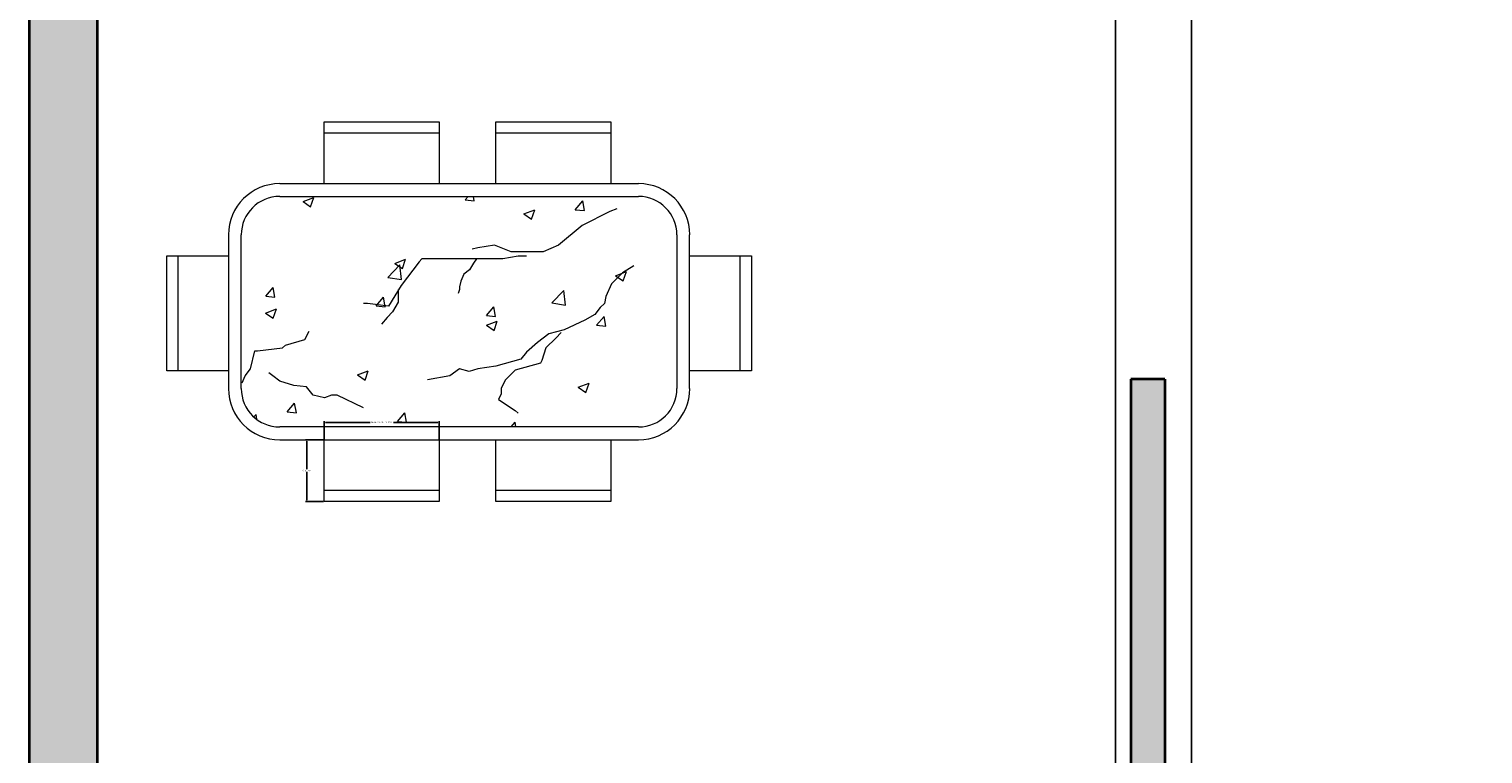
# Model space of a CAD drawing. Units: inches. Extents: x -5 to 366, y -496 to 54.
# Tile 8 of 10: x 22 to 214, y -205 to -110. Entities that reach past the tile are written whole.
import ezdxf

# ---------------------------------------------------------------- set-up
doc = ezdxf.new("R2010")
doc.units = ezdxf.units.IN
doc.header["$MEASUREMENT"] = 0
for name, color, linetype, lineweight in [('A-ANNO-DIMS', 2, 'Continuous', 18), ('A-FURN', 8, 'Continuous', 18), ('A-WALL', 7, 'Continuous', 35), ('A-WALL-PATT', 252, 'Continuous', 13)]:
    doc.layers.add(name, color=color, linetype=linetype, lineweight=lineweight)
doc.styles.get("Standard").update_dxf_attribs({"font": 'arial.ttf'})
doc.dimstyles.get("Standard").update_dxf_attribs({"dimtxt": 0.18, "dimasz": 0.18, "dimexe": 0.18, "dimexo": 0.0625, "dimgap": 0.09, "dimtad": 0, "dimtih": 1, "dimtoh": 1, "dimdec": 0, "dimzin": 0, "dimdsep": 46, "dimlunit": 3, "dimtxsty": 'Standard', "dimcen": 0.09, "dimadec": 0, "dimazin": 0, "dimtfac": 1, "dimtdec": 0, "dimtofl": 0, "dimtmove": 0, "dimatfit": 3, "dimfxl": 1, "dimtolj": 1, "dimtzin": 0, "dimarcsym": 0})

# ---------------------------------------------------------------- blocks, each defined once
blk = doc.blocks.new('CHAIR-DINING')
for p, q in [((0, 0), (0, 8.16)), ((0, 8.16), (15.22, 8.16)), ((15.22, 8.16), (15.22, 0)), ((15.22, 6.67), (0, 6.67))]:
    blk.add_line(p, q)
blk = doc.blocks.new('*D13')
at = {"layer": 'A-ANNO-DIMS', "color": 0, "lineweight": -2, "transparency": 16777216}
for p, q in [((60.89, -163.78), (60.89, -161.38)), ((61.07, -161.56), (66.97, -161.56)), ((75.93, -161.56), (70.04, -161.56)), ((76.11, -163.78), (76.11, -161.38))]:
    blk.add_line(p, q, dxfattribs=at)
at = {"layer": 'A-ANNO-DIMS', "color": 0, "transparency": 16777216}
for points in [[(61.07, -161.53), (61.07, -161.59), (60.89, -161.56)], [(75.93, -161.53), (75.93, -161.59), (76.11, -161.56)]]:
    blk.add_solid(points, dxfattribs=at)
at = {"layer": 'Defpoints', "color": 0, "transparency": 16777216}
for p in [(60.89, -161.56), (60.89, -163.84), (76.11, -163.84)]:
    blk.add_point(p, dxfattribs=at)
at = {"layer": 'A-ANNO-DIMS', "color": 0, "transparency": 16777216, "insert": (68.5, -161.56), "char_height": 0.18, "attachment_point": 5}
blk.add_mtext('\\A1;DINING CHAIR 1\'-3" TYP.', dxfattribs=at)
blk = doc.blocks.new('*D14')
at = {"layer": 'A-ANNO-DIMS', "color": 0, "lineweight": -2, "transparency": 16777216}
for p, q in [((60.83, -163.84), (58.42, -163.84)), ((58.6, -164.02), (58.6, -167.74)), ((58.6, -171.82), (58.6, -168.1)), ((60.83, -172), (58.42, -172))]:
    blk.add_line(p, q, dxfattribs=at)
at = {"layer": 'A-ANNO-DIMS', "color": 0, "transparency": 16777216}
for points in [[(58.57, -164.02), (58.63, -164.02), (58.6, -163.84)], [(58.57, -171.82), (58.63, -171.82), (58.6, -172)]]:
    blk.add_solid(points, dxfattribs=at)
at = {"layer": 'Defpoints', "color": 0, "transparency": 16777216}
for p in [(60.89, -163.84), (58.6, -172), (60.89, -172)]:
    blk.add_point(p, dxfattribs=at)
at = {"layer": 'A-ANNO-DIMS', "color": 0, "transparency": 16777216, "insert": (58.6, -167.92), "char_height": 0.18, "attachment_point": 5}
blk.add_mtext('\\A1;0\'-8" TYP.', dxfattribs=at)
blk = doc.blocks.new('*D29')
at = {"layer": 'A-ANNO-DIMS', "color": 0, "lineweight": -2, "transparency": 16777216}
for p, q in [((165.43, -380.42), (165.43, 53.15)), ((165.61, 52.97), (170.03, 52.97)), ((175.25, 52.97), (170.83, 52.97)), ((175.43, -380.42), (175.43, 53.15))]:
    blk.add_line(p, q, dxfattribs=at)
at = {"layer": 'A-ANNO-DIMS', "color": 0, "transparency": 16777216}
for points in [[(165.61, 53), (165.61, 52.94), (165.43, 52.97)], [(175.25, 53), (175.25, 52.94), (175.43, 52.97)]]:
    blk.add_solid(points, dxfattribs=at)
at = {"layer": 'Defpoints', "color": 0, "transparency": 16777216}
for p in [(175.43, 52.97), (165.43, -380.48), (175.43, -380.48)]:
    blk.add_point(p, dxfattribs=at)
at = {"layer": 'A-ANNO-DIMS', "color": 0, "transparency": 16777216, "insert": (170.43, 52.97), "char_height": 0.18, "attachment_point": 5}
blk.add_mtext('\\A1;0\'-10"', dxfattribs=at)

msp = doc.modelspace()

# ---------------------------------------------------------------- hatches: boundary and pattern name
at = {"layer": 'A-WALL-PATT'}
h = msp.add_hatch(color=256, dxfattribs=at)
h.dxf.hatch_style = 1
h.paths.add_polyline_path([(324.93, 26.52), (21.93, 26.52), (21.93, -456.98), (26.43, -456.98), (26.43, -331.98), (30.93, -331.98), (30.93, -322.98), (30.93, -106.98), (110.93, -106.98), (110.93, -104.73), (110.93, -102.48), (30.93, -102.48), (30.93, 17.52), (138.93, 17.52), (141.18, 17.52), (143.43, 17.52), (183.43, 17.52), (187.93, 17.52), (315.93, 17.52), (315.93, -102.48), (315.93, -106.98), (315.93, -255.48), (171.93, -255.48), (171.93, -155.84), (167.43, -155.84), (167.43, -291.98), (171.93, -291.98), (171.93, -259.98), (315.93, -259.98), (315.93, -375.98), (297.93, -375.98), (297.93, -380.48), (315.93, -380.48), (315.93, -452.48), (315.93, -456.98), (324.93, -456.98)])
h.paths.add_polyline_path([(143.43, -18.48), (143.43, -13.98), (138.93, -13.98), (138.93, -106.98), (187.93, -106.98), (187.93, -102.48), (143.43, -102.48)], flags=17)

# ---------------------------------------------------------------- linework, layer by layer
at = {"layer": 'A-FURN'}
for p, q in [((102.41, -130.01), (55.03, -130.01)), ((55.03, -131.7), (102.41, -131.7)), ((58.11, -132.38), (59.53, -131.83)), ((58.11, -132.38), (59.12, -133.06)), ((59.12, -133.06), (59.53, -131.83)), ((79.51, -132.16), (79.9, -131.7)), ((79.51, -132.16), (80.72, -132.27)), ((80.72, -132.27), (80.62, -131.7)), ((94.07, -133.44), (95.05, -132.27)), ((95.28, -133.55), (95.05, -132.27)), ((87.28, -134), (88.71, -133.46)), ((87.28, -134), (88.29, -134.68)), ((88.29, -134.68), (88.71, -133.46)), ((94.07, -133.44), (95.28, -133.54)), ((98.65, -133.7), (94.97, -135.54)), ((99.57, -133.34), (98.65, -133.7)), ((94.97, -135.54), (91.85, -138.11)), ((48.27, -136.77), (48.27, -157.08)), ((49.96, -157.08), (49.96, -136.77)), ((83.38, -138.11), (81.18, -138.48)), ((85.59, -139.03), (83.38, -138.11)), ((91.85, -138.11), (89.82, -139.03)), ((107.48, -136.77), (107.48, -157.08)), ((109.17, -157.08), (109.17, -136.77)), ((70.23, -140.55), (71.65, -140)), ((71.24, -141.23), (71.65, -140)), ((73.82, -139.95), (73.45, -140.32)), ((84.49, -139.95), (73.82, -139.95)), ((81.18, -138.48), (80.44, -138.67)), ((81, -139.94), (80.63, -140.5)), ((86.51, -139.58), (84.49, -139.95)), ((89.82, -139.03), (85.59, -139.03)), ((87.62, -139.58), (86.51, -139.58)), ((69.31, -142.39), (70.9, -140.75)), ((70.23, -140.55), (71.24, -141.23)), ((71.12, -142.68), (70.9, -140.75)), ((73.45, -140.32), (71.06, -143.44)), ((79.34, -141.97), (78.97, -142.88)), ((80.08, -141.41), (79.34, -141.97)), ((80.63, -140.5), (80.08, -141.41)), ((100.31, -141.79), (98.84, -143.26)), ((99.4, -142.18), (100.83, -141.63)), ((101.78, -140.87), (100.31, -141.79)), ((100.41, -142.86), (100.83, -141.63)), ((53.2, -144.89), (54.18, -143.72)), ((54.41, -145), (54.18, -143.72)), ((69.31, -142.39), (71.12, -142.67)), ((71.06, -143.44), (69.4, -146.2)), ((70.69, -143.99), (70.69, -145.65)), ((78.79, -143.99), (78.6, -144.54)), ((78.97, -142.88), (78.79, -143.62)), ((78.79, -143.62), (78.79, -143.99)), ((98.84, -143.26), (98.1, -144.91)), ((99.4, -142.18), (100.41, -142.86)), ((53.2, -144.89), (54.41, -144.99)), ((66.64, -145.83), (66.09, -145.83)), ((69.4, -146.2), (66.64, -145.83)), ((67.76, -146.16), (68.74, -145)), ((68.98, -146.27), (68.74, -145)), ((70.69, -145.65), (69.95, -146.93)), ((90.98, -145.76), (92.56, -144.11)), ((90.98, -145.76), (92.79, -146.04)), ((92.79, -146.04), (92.56, -144.11)), ((97.92, -145.83), (97.37, -146.38)), ((98.1, -144.91), (97.92, -145.83)), ((53.17, -147.1), (54.59, -146.55)), ((53.17, -147.1), (54.18, -147.78)), ((54.18, -147.78), (54.59, -146.55)), ((67.76, -146.16), (68.98, -146.27)), ((69.22, -147.67), (68.48, -148.59)), ((69.95, -146.93), (69.22, -147.67)), ((82.33, -147.44), (83.3, -146.27)), ((82.33, -147.44), (83.54, -147.54)), ((83.54, -147.54), (83.3, -146.27)), ((96.63, -147.3), (95.34, -148.04)), ((97.37, -146.38), (96.63, -147.3)), ((96.89, -148.71), (97.87, -147.54)), ((98.1, -148.82), (97.87, -147.54)), ((58.36, -150.61), (58.92, -149.51)), ((82.35, -148.72), (83.77, -148.18)), ((82.35, -148.72), (83.35, -149.4)), ((83.36, -149.41), (83.77, -148.18)), ((92.58, -149.32), (90.56, -149.87)), ((92.21, -149.69), (91.48, -150.43)), ((95.34, -148.04), (92.58, -149.32)), ((96.89, -148.71), (98.1, -148.82)), ((55.42, -151.71), (55.79, -151.34)), ((55.79, -151.34), (58.36, -150.61)), ((89.09, -150.98), (87.62, -152.26)), ((90.56, -149.87), (89.09, -150.98)), ((91.48, -150.43), (90.19, -151.71)), ((51.19, -154.47), (51.74, -152.08)), ((51.74, -152.08), (52.11, -152.08)), ((52.11, -152.08), (55.42, -151.71)), ((86.88, -153.18), (83.57, -154.1)), ((87.62, -152.26), (86.88, -153.18)), ((89.64, -153.37), (89.46, -153.73)), ((90.19, -151.71), (89.64, -153.37)), ((50.09, -156.31), (50.45, -155.39)), ((50.45, -155.39), (51.19, -154.47)), ((54.14, -155.38), (53.58, -155.01)), ((55.06, -156.12), (54.14, -155.38)), ((65.29, -155.27), (66.71, -154.73)), ((65.29, -155.27), (66.3, -155.95)), ((66.3, -155.95), (66.71, -154.73)), ((77.5, -155.39), (74.55, -155.94)), ((78.79, -154.47), (77.5, -155.39)), ((80.07, -154.84), (78.79, -154.47)), ((81.18, -154.47), (80.07, -154.84)), ((83.57, -154.1), (81.18, -154.47)), ((86.14, -154.65), (84.86, -155.94)), ((89.46, -153.73), (86.14, -154.65)), ((56.9, -156.67), (55.06, -156.12)), ((58.55, -156.85), (56.9, -156.67)), ((59.47, -157.95), (58.55, -156.85)), ((84.86, -155.94), (84.3, -157.04)), ((84.3, -157.04), (84.3, -157.78)), ((94.46, -156.9), (95.89, -156.35)), ((94.46, -156.9), (95.47, -157.58)), ((95.47, -157.58), (95.89, -156.35)), ((56.02, -160.16), (57, -158.99)), ((57.23, -160.27), (57, -158.99)), ((60.94, -158.32), (59.47, -157.95)), ((61.86, -157.95), (60.94, -158.32)), ((62.6, -157.95), (61.86, -157.95)), ((66.09, -159.61), (62.6, -157.95)), ((84.3, -157.78), (83.94, -158.51)), ((83.94, -158.51), (86.14, -159.98)), ((51.62, -160.83), (51.92, -160.52)), ((51.99, -161.14), (51.92, -160.52)), ((56.02, -160.16), (57.23, -160.27)), ((70.58, -161.43), (71.56, -160.27)), ((71.79, -161.54), (71.56, -160.27)), ((86.14, -159.98), (86.51, -160.35)), ((102.41, -162.15), (55.03, -162.15)), ((70.58, -161.43), (71.79, -161.54)), ((85.61, -162.15), (86.12, -161.54)), ((86.23, -162.15), (86.12, -161.54)), ((55.03, -163.84), (102.41, -163.84))]:
    msp.add_line(p, q, dxfattribs=at)
for centre, radius, start, end in [((55.03, -136.77), 6.77, 90, 180), ((102.41, -136.77), 6.77, 0, 90), ((55.03, -136.77), 5.08, 90, 180), ((102.41, -136.77), 5.08, 0, 90), ((55.03, -157.08), 6.77, 180, 270), ((55.03, -157.08), 5.08, 180, 270), ((102.41, -157.08), 5.08, 270, 0), ((102.41, -157.08), 6.77, 270, 0)]:
    msp.add_arc(centre, radius, start, end, dxfattribs=at)
at = {"layer": 'A-WALL'}
for p, q in [((21.93, 26.52), (21.93, -456.98)), ((30.93, -106.98), (30.93, -322.98)), ((167.43, -155.84), (167.43, -291.98)), ((171.93, -155.84), (167.43, -155.84)), ((171.93, -155.84), (171.93, -255.48))]:
    msp.add_line(p, q, dxfattribs=at)

# ---------------------------------------------------------------- block references
at = {"layer": 'A-FURN'}
for p in [(60.89, -130.01), (83.56, -130.01)]:
    msp.add_blockref('CHAIR-DINING', p, dxfattribs=at)
for p, rotation in [((48.27, -154.74), 89.99999999673713), ((109.17, -139.52), 269.9999999872913), ((76.11, -163.84), 180), ((98.78, -163.84), 180)]:
    msp.add_blockref('CHAIR-DINING', p, dxfattribs=dict(at, rotation=rotation))

# ---------------------------------------------------------------- dimensions: what is measured, and where the dimension line sits
at = {"layer": 'A-ANNO-DIMS'}
dim = msp.add_linear_dim(base=(175.43, 52.97), p1=(165.43, -380.48), p2=(175.43, -380.48), dimstyle='Standard', override={"dimdec": 1, "dimlfac": 1, "dimrnd": 0, "dimzin": 1, "dimdsep": 46, "dimlunit": 4, "dimfrac": 2}, dxfattribs=at)
dim.commit()
dim.dimension.update_dxf_attribs({"geometry": '*D29', "text_midpoint": (170.43, 52.97)})
for base, p1, p2, angle, text, picture, middle in [((60.89, -161.56), (76.11, -163.84), (60.89, -163.84), 180, 'DINING CHAIR <> TYP.', '*D13', (68.5, -161.56)), ((58.6, -172), (60.89, -163.84), (60.89, -172), 270, '<> TYP.', '*D14', (58.6, -167.92))]:
    dim = msp.add_linear_dim(base=base, p1=p1, p2=p2, angle=angle, text=text, dimstyle='Standard', override={"dimdec": 1, "dimlfac": 1, "dimrnd": 0, "dimzin": 1, "dimdsep": 46, "dimlunit": 4, "dimfrac": 2}, dxfattribs=at)
    dim.commit()
    dim.dimension.update_dxf_attribs({"geometry": picture, "text_midpoint": middle})

doc.saveas('drawing.dxf')
